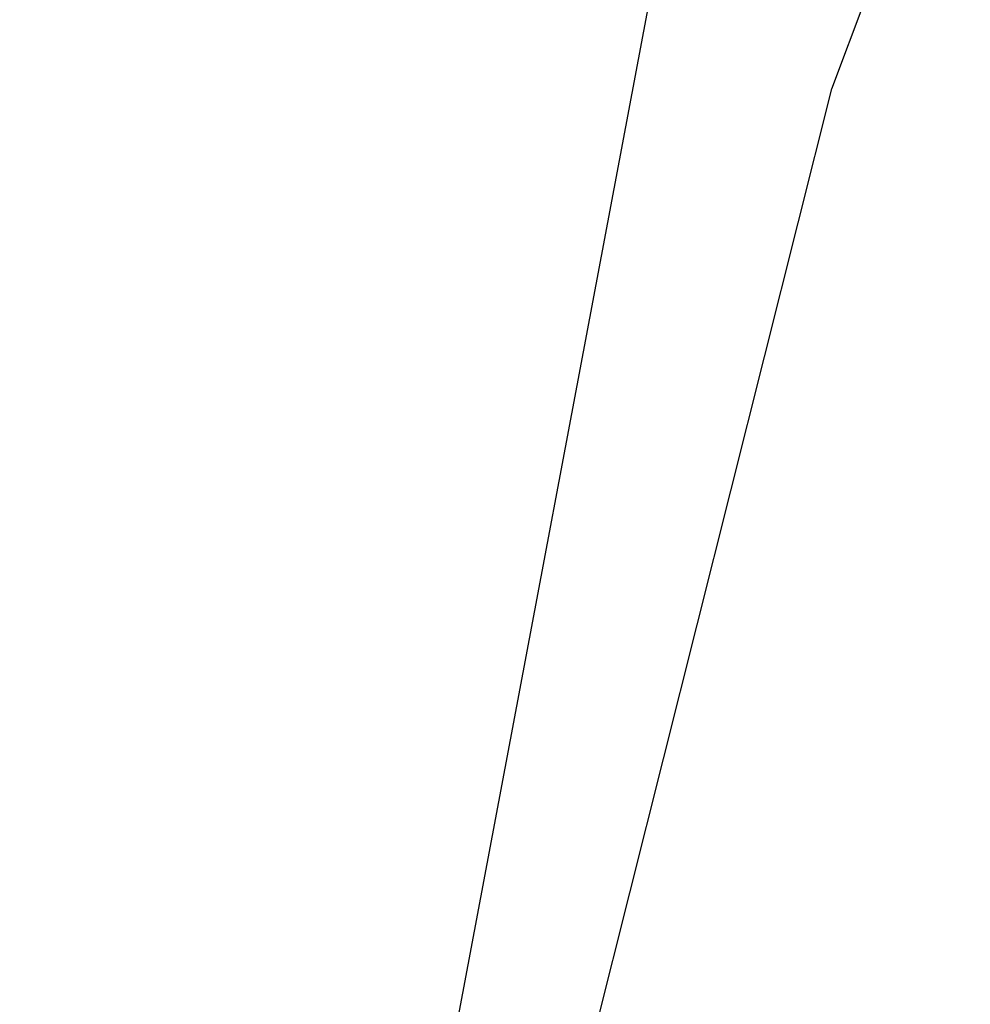
# Model space of a CAD drawing. Units: inches. Extents: x 3590 to 5167, y 65 to 1917.
# Tile 82 of 100: x 5051.162 to 5051.6658, y 1788.0928 to 1788.6144. Entities that reach past the tile are written whole.
import ezdxf

# ---------------------------------------------------------------- set-up
doc = ezdxf.new("R2010")
doc.units = ezdxf.units.IN
doc.layers.add('A-ANNO-DIMS', color=2, linetype='Continuous', lineweight=18)
doc.layers.add('L-PLNT', color=94, linetype='Continuous', lineweight=18)
doc.layers.add('DIENHOA', color=3, linetype='Continuous')
doc.styles.get("Standard").update_dxf_attribs({"font": 'arial.ttf'})
doc.dimstyles.new('ISO-25', dxfattribs={"dimtxt": 9, "dimasz": 2.5, "dimexe": 1.25, "dimexo": 0.625, "dimtad": 1, "dimdec": 1, "dimlunit": 3, "dimtxsty": 'Standard', "dimcen": 2.5, "dimadec": 0, "dimazin": 0, "dimtfac": 1, "dimtdec": 1, "dimtmove": 0, "dimatfit": 3, "dimfxl": 1, "dimarcsym": 0})

# ---------------------------------------------------------------- blocks, each defined once
blk = doc.blocks.new('Cay03_mb')
at = {"layer": 'DIENHOA'}
for points in [[(87.915, 628.525), (75.456, 544.179), (61.266, 461.155), (46.129, 379.14), (30.826, 297.822), (16.139, 216.889), (2.853, 136.026), (-8.252, 54.923), (-16.392, -26.735)], [(23.687, -5.439), (19.839, 92.987), (20.283, 176.968), (25.016, 248.547), (34.033, 309.769), (47.331, 362.677), (64.906, 409.313), (86.753, 451.722), (112.868, 491.948)]]:
    blk.add_lwpolyline(points, dxfattribs=at)
blk = doc.blocks.new('*D322')
at = {"layer": 'A-ANNO-DIMS', "color": 0, "lineweight": -2, "transparency": 16777216}
for p, q in [((5035.74373, 1766.18424), (5035.74373, 1761.19899)), ((5064.81203, 1766.18424), (5064.81203, 1761.19899)), ((5038.24373, 1762.44899), (5062.31203, 1762.44899)), ((5064.81203, 1762.44899), (5166.99109, 1762.44899))]:
    blk.add_line(p, q, dxfattribs=at)
at = {"layer": 'A-ANNO-DIMS', "color": 0, "transparency": 16777216}
for points in [[(5038.24373, 1762.86566), (5038.24373, 1762.03233), (5035.74373, 1762.44899)], [(5062.31203, 1762.86566), (5062.31203, 1762.03233), (5064.81203, 1762.44899)]]:
    blk.add_solid(points, dxfattribs=at)
at = {"layer": 'Defpoints', "color": 0, "transparency": 16777216}
for p in [(5035.74373, 1766.80924), (5064.81203, 1766.80924), (5064.81203, 1762.44899)]:
    blk.add_point(p, dxfattribs=at)
at = {"layer": 'A-ANNO-DIMS', "color": 0, "transparency": 16777216, "insert": (5117.15156, 1767.66915), "char_height": 9, "attachment_point": 5}
blk.add_mtext('PLANT 2\'-5" TYP.', dxfattribs=at)

msp = doc.modelspace()

# ---------------------------------------------------------------- block references
at = {"layer": 'L-PLNT', "xscale": 0.0245452446402784, "yscale": 0.0245452446402784, "zscale": 0.0245452446402784}
msp.add_blockref('Cay03_mb', (5050.43062, 1779.67584), dxfattribs=at)

# ---------------------------------------------------------------- dimensions: what is measured, and where the dimension line sits
at = {"layer": 'A-ANNO-DIMS'}
dim = msp.add_linear_dim(base=(5064.81203, 1762.44899), p1=(5035.74373, 1766.80924), p2=(5064.81203, 1766.80924), text='PLANT <> TYP.', dimstyle='ISO-25', override={"dimdec": 1, "dimlfac": 1, "dimrnd": 0, "dimzin": 1, "dimdsep": 46, "dimlunit": 4, "dimfrac": 2}, dxfattribs=at)
dim.commit()
dim.dimension.update_dxf_attribs({"geometry": '*D322', "text_midpoint": (5117.15156, 1767.66915)})

doc.saveas('drawing.dxf')
